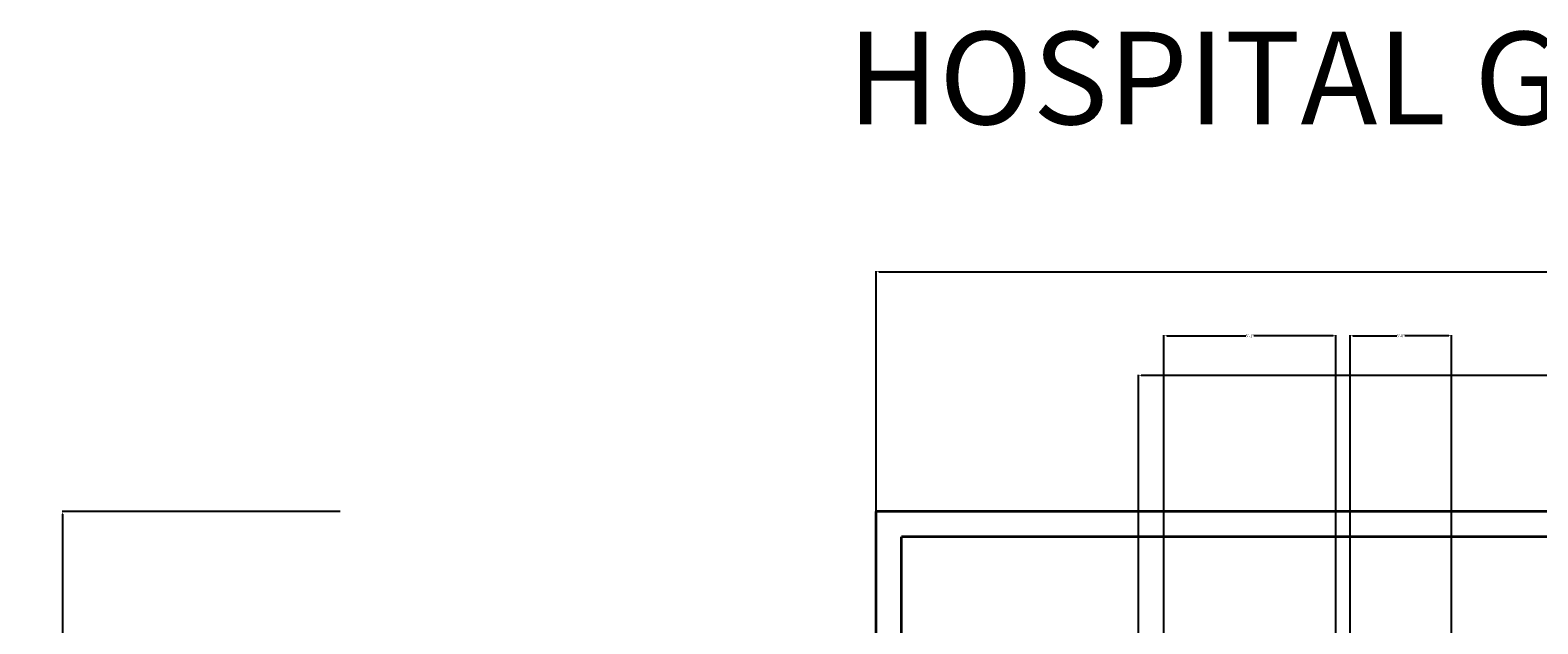
# Model space of a CAD drawing. Units: inches. Extents: x -364 to 705, y -52 to 1250.
# Tile 26 of 34: x -364 to 170, y 1039 to 1250. Entities that reach past the tile are written whole.
import ezdxf

# ---------------------------------------------------------------- set-up
doc = ezdxf.new("R2010")
doc.units = ezdxf.units.IN
doc.header["$MEASUREMENT"] = 0
for name, color, linetype, lineweight in [('A-ANNO-DIMS', 4, 'Continuous', 18), ('A-ANNO-TITL', 6, 'Continuous', 35), ('C-WALL', 41, 'Continuous', 35)]:
    doc.layers.add(name, color=color, linetype=linetype, lineweight=lineweight)
doc.styles.get("Standard").update_dxf_attribs({"font": 'arial.ttf'})
doc.dimstyles.get("Standard").update_dxf_attribs({"dimtxt": 1, "dimasz": 1, "dimexe": 0.18, "dimexo": 0.0625, "dimgap": 0.09, "dimtad": 0, "dimtih": 1, "dimtoh": 1, "dimdec": 0, "dimzin": 0, "dimdsep": 46, "dimlunit": 3, "dimtxsty": 'Standard', "dimcen": 0.09, "dimadec": 0, "dimazin": 0, "dimtfac": 1, "dimtdec": 0, "dimtofl": 0, "dimtmove": 0, "dimatfit": 3, "dimfxl": 1, "dimtolj": 1, "dimtzin": 0, "dimarcsym": 0})

# ---------------------------------------------------------------- blocks, each defined once
blk = doc.blocks.new('*D18')
at = {"layer": 'A-ANNO-DIMS', "color": 0, "lineweight": -2, "transparency": 16777216}
for p, q in [((-254.46, 1079.11), (-353.05, 1079.11)), ((-352.87, 1078.11), (-352.87, 551.84)), ((-352.87, 12.11), (-352.87, 538.39)), ((-254.46, 11.11), (-353.05, 11.11))]:
    blk.add_line(p, q, dxfattribs=at)
at = {"layer": 'A-ANNO-DIMS', "color": 0, "transparency": 16777216}
for points in [[(-353.04, 1078.11), (-352.7, 1078.11), (-352.87, 1079.11)], [(-353.04, 12.11), (-352.7, 12.11), (-352.87, 11.11)]]:
    blk.add_solid(points, dxfattribs=at)
at = {"layer": 'Defpoints', "color": 0, "transparency": 16777216}
for p in [(-254.4, 1079.11), (-352.87, 11.11), (-254.4, 11.11)]:
    blk.add_point(p, dxfattribs=at)
at = {"layer": 'A-ANNO-DIMS', "color": 0, "transparency": 16777216, "insert": (-352.87, 545.11), "char_height": 1, "width": 1.6985, "attachment_point": 5}
blk.add_mtext("\\A1;{\\H13x;89'}", dxfattribs=at)
blk = doc.blocks.new('*D22')
at = {"layer": 'A-ANNO-DIMS', "color": 0, "lineweight": -2, "transparency": 16777216}
for p, q in [((-64.42, 1079.18), (-64.42, 1164.27)), ((-63.42, 1164.09), (265.66, 1164.09)), ((639.58, 1164.09), (310.5, 1164.09)), ((640.58, 1079.18), (640.58, 1164.27))]:
    blk.add_line(p, q, dxfattribs=at)
at = {"layer": 'A-ANNO-DIMS', "color": 0, "transparency": 16777216}
for points in [[(-63.42, 1164.26), (-63.42, 1163.93), (-64.42, 1164.09)], [(639.58, 1164.26), (639.58, 1163.93), (640.58, 1164.09)]]:
    blk.add_solid(points, dxfattribs=at)
at = {"layer": 'Defpoints', "color": 0, "transparency": 16777216}
for p in [(640.58, 1164.09), (-64.42, 1079.11), (640.58, 1079.11)]:
    blk.add_point(p, dxfattribs=at)
at = {"layer": 'A-ANNO-DIMS', "color": 0, "transparency": 16777216, "insert": (288.08, 1164.09), "char_height": 1, "attachment_point": 5}
blk.add_mtext('\\A1;{\\H13x;58\'-9"}', dxfattribs=at)
blk = doc.blocks.new('*D23')
at = {"layer": 'A-ANNO-DIMS', "color": 0, "lineweight": -2, "transparency": 16777216}
for p, q in [((28.58, 986.18), (28.58, 1127.53)), ((29.58, 1127.35), (265.4, 1127.35)), ((546.58, 1127.35), (310.76, 1127.35)), ((547.58, 986.18), (547.58, 1127.53))]:
    blk.add_line(p, q, dxfattribs=at)
at = {"layer": 'A-ANNO-DIMS', "color": 0, "transparency": 16777216}
for points in [[(29.58, 1127.52), (29.58, 1127.18), (28.58, 1127.35)], [(546.58, 1127.52), (546.58, 1127.18), (547.58, 1127.35)]]:
    blk.add_solid(points, dxfattribs=at)
at = {"layer": 'Defpoints', "color": 0, "transparency": 16777216}
for p in [(547.58, 1127.35), (28.58, 986.11), (547.58, 986.11)]:
    blk.add_point(p, dxfattribs=at)
at = {"layer": 'A-ANNO-DIMS', "color": 0, "transparency": 16777216, "insert": (288.08, 1127.35), "char_height": 1, "attachment_point": 5}
blk.add_mtext('\\A1;{\\H13x;43\'-3"}', dxfattribs=at)
blk = doc.blocks.new('*D91')
at = {"layer": 'A-ANNO-DIMS', "color": 0, "lineweight": -2, "transparency": 16777216}
for p, q in [((37.58, 977.18), (37.58, 1141.54)), ((38.58, 1141.36), (66.66, 1141.36)), ((97.58, 1141.36), (69.5, 1141.36)), ((98.58, 977.18), (98.58, 1141.54))]:
    blk.add_line(p, q, dxfattribs=at)
at = {"layer": 'A-ANNO-DIMS', "color": 0, "transparency": 16777216}
for points in [[(38.58, 1141.53), (38.58, 1141.2), (37.58, 1141.36)], [(97.58, 1141.53), (97.58, 1141.2), (98.58, 1141.36)]]:
    blk.add_solid(points, dxfattribs=at)
at = {"layer": 'Defpoints', "color": 0, "transparency": 16777216}
for p in [(98.58, 1141.36), (37.58, 977.11), (98.58, 977.11)]:
    blk.add_point(p, dxfattribs=at)
at = {"layer": 'A-ANNO-DIMS', "color": 0, "transparency": 16777216, "insert": (68.08, 1141.36), "char_height": 1, "attachment_point": 5}
blk.add_mtext('\\A1;5\'-1"', dxfattribs=at)
blk = doc.blocks.new('*D92')
at = {"layer": 'A-ANNO-DIMS', "color": 0, "lineweight": -2, "transparency": 16777216}
for p, q in [((103.58, 977.18), (103.58, 1141.54)), ((104.58, 1141.36), (120.16, 1141.36)), ((138.58, 1141.36), (123, 1141.36)), ((139.58, 977.18), (139.58, 1141.54))]:
    blk.add_line(p, q, dxfattribs=at)
at = {"layer": 'A-ANNO-DIMS', "color": 0, "transparency": 16777216}
for points in [[(104.58, 1141.53), (104.58, 1141.2), (103.58, 1141.36)], [(138.58, 1141.53), (138.58, 1141.2), (139.58, 1141.36)]]:
    blk.add_solid(points, dxfattribs=at)
at = {"layer": 'Defpoints', "color": 0, "transparency": 16777216}
for p in [(139.58, 1141.36), (103.58, 977.11), (139.58, 977.11)]:
    blk.add_point(p, dxfattribs=at)
at = {"layer": 'A-ANNO-DIMS', "color": 0, "transparency": 16777216, "insert": (121.58, 1141.36), "char_height": 1, "attachment_point": 5}
blk.add_mtext('\\A1;3\'-0"', dxfattribs=at)

msp = doc.modelspace()

# ---------------------------------------------------------------- linework, layer by layer
at = {"layer": 'C-WALL'}
for p, q in [((640.58, 1079.11), (-64.42, 1079.11)), ((-64.42, 11.11), (-64.42, 1079.11)), ((631.58, 1070.11), (-55.42, 1070.11)), ((-55.42, 11.11), (-55.42, 1070.11))]:
    msp.add_line(p, q, dxfattribs=at)

# ---------------------------------------------------------------- texts
at = {"layer": 'A-ANNO-TITL', "insert": (-74.72, 1249.15), "char_height": 32.815, "attachment_point": 1}
msp.add_mtext_dynamic_manual_height_columns('HOSPITAL GROUND FLOOR PLAN ', width=1304.1967, gutter_width=2.52, heights=[0], dxfattribs=at)

# ---------------------------------------------------------------- dimensions: what is measured, and where the dimension line sits
at = {"layer": 'A-ANNO-DIMS'}
for base, p1, p2, picture, middle in [((640.58, 1164.09), (-64.42, 1079.11), (640.58, 1079.11), '*D22', (288.08, 1164.09)), ((547.58, 1127.35), (28.58, 986.11), (547.58, 986.11), '*D23', (288.08, 1127.35))]:
    dim = msp.add_linear_dim(base=base, p1=p1, p2=p2, text='{\\H13x;<>}', dimstyle='Standard', override={"dimclrd": 0, "dimclre": 0, "dimclrt": 0}, dxfattribs=at)
    dim.commit()
    dim.dimension.update_dxf_attribs({"geometry": picture, "text_midpoint": middle})
for base, p1, p2, picture, middle in [((98.58, 1141.36), (37.58, 977.11), (98.58, 977.11), '*D91', (68.08, 1141.36)), ((139.58, 1141.36), (103.58, 977.11), (139.58, 977.11), '*D92', (121.58, 1141.36))]:
    dim = msp.add_linear_dim(base=base, p1=p1, p2=p2, dimstyle='Standard', override={"dimdec": 1, "dimlfac": 1, "dimrnd": 0, "dimzin": 1, "dimdsep": 46, "dimlunit": 4, "dimfrac": 2}, dxfattribs=at)
    dim.commit()
    dim.dimension.update_dxf_attribs({"geometry": picture, "text_midpoint": middle})
dim = msp.add_linear_dim(base=(-352.87, 11.11), p1=(-254.4, 1079.11), p2=(-254.4, 11.11), angle=90, text='{\\H13x;<>}', dimstyle='Standard', override={"dimclrd": 0, "dimclre": 0, "dimclrt": 0}, dxfattribs=at)
dim.commit()
dim.dimension.update_dxf_attribs({"geometry": '*D18', "text_midpoint": (-352.87, 545.11)})

doc.saveas('drawing.dxf')
